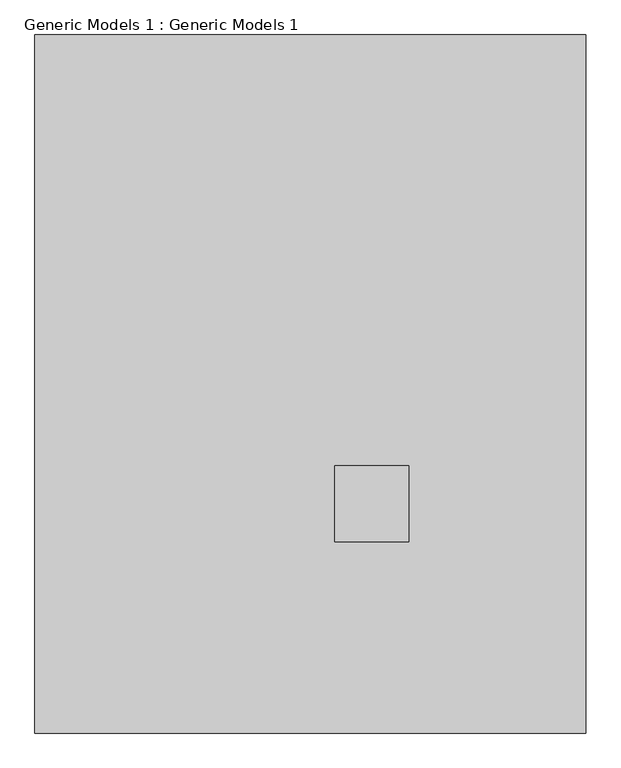
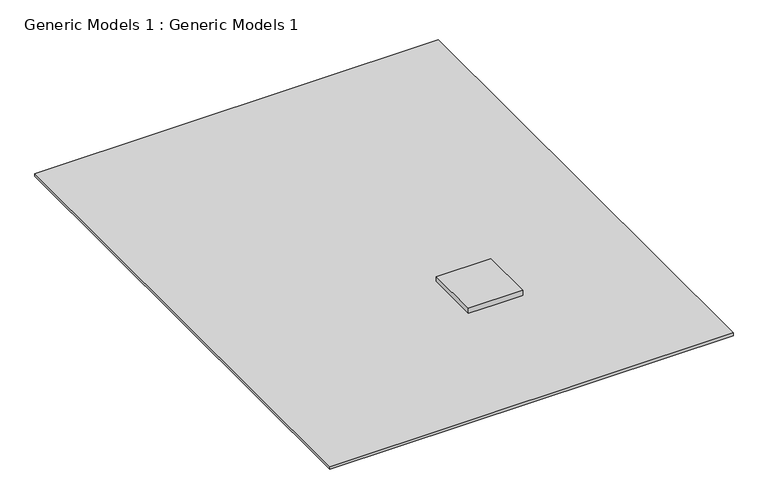
"""IFC4 building model written with IfcOpenShell, lengths in millimetres: proxy geometry, Generic Models 1 : Generic Models 1."""

from ifc_helpers import new_model, si_unit, frame, origin, origin_with_axes, place, context, project, spatial, polyline, outline, extrude, source, transform, mapped, element, save


def generic_models_1_generic_models_1_92a5afb8(model_context):
    return source(origin(), model_context, "Body", "SweptSolid", [
        extrude(outline(polyline([(-5387.0886697, 8901.6694682), (-5387.0886697, -20177.6638993), (-28339.6856653, -20177.6638993), (-28339.6856653, 8901.6694682), (-5387.0886697, 8901.6694682)])), frame((0.0, 0.0, -152.4), z_axis=(0.0, 0.0, 1.0), x_axis=(1.0, 0.0, 0.0)), (0.0, 0.0, 1.0), 152.4),
        extrude(outline(polyline([(-12759.4386697, -9042.3511954), (-12759.4386697, -12204.6511954), (-15845.5386697, -12204.6511954), (-15845.5386697, -9042.3511954), (-12759.4386697, -9042.3511954)])), origin_with_axes(), (0.0, 0.0, 1.0), 304.8),
    ])


if __name__ == "__main__":
    model = new_model("IFC4")
    model_context = context("Model", 3, world=origin())
    ifc_project = project(units=[si_unit("LENGTHUNIT", "METRE", prefix="MILLI")], contexts=[model_context])
    site = spatial("IfcSite", under=ifc_project)
    building = spatial("IfcBuilding", under=site)
    placement = place(None, origin())
    generic_models_1_generic_models_1_shape = generic_models_1_generic_models_1_92a5afb8(model_context)
    element("IfcBuildingElementProxy", 1, Name="Generic Models 1 : Generic Models 1", ObjectType="Generic Models 1 : Generic Models 1", at=placement, inside=building, context=model_context, shape_type="MappedRepresentation", body=[
        mapped(generic_models_1_generic_models_1_shape, transform((0.0, 0.0, 0.0), x_axis=(1.0, 0.0, 0.0), y_axis=(0.0, 1.0, 0.0), z_axis=(0.0, 0.0, 1.0))),
    ])
    save(model, "model.ifc")
